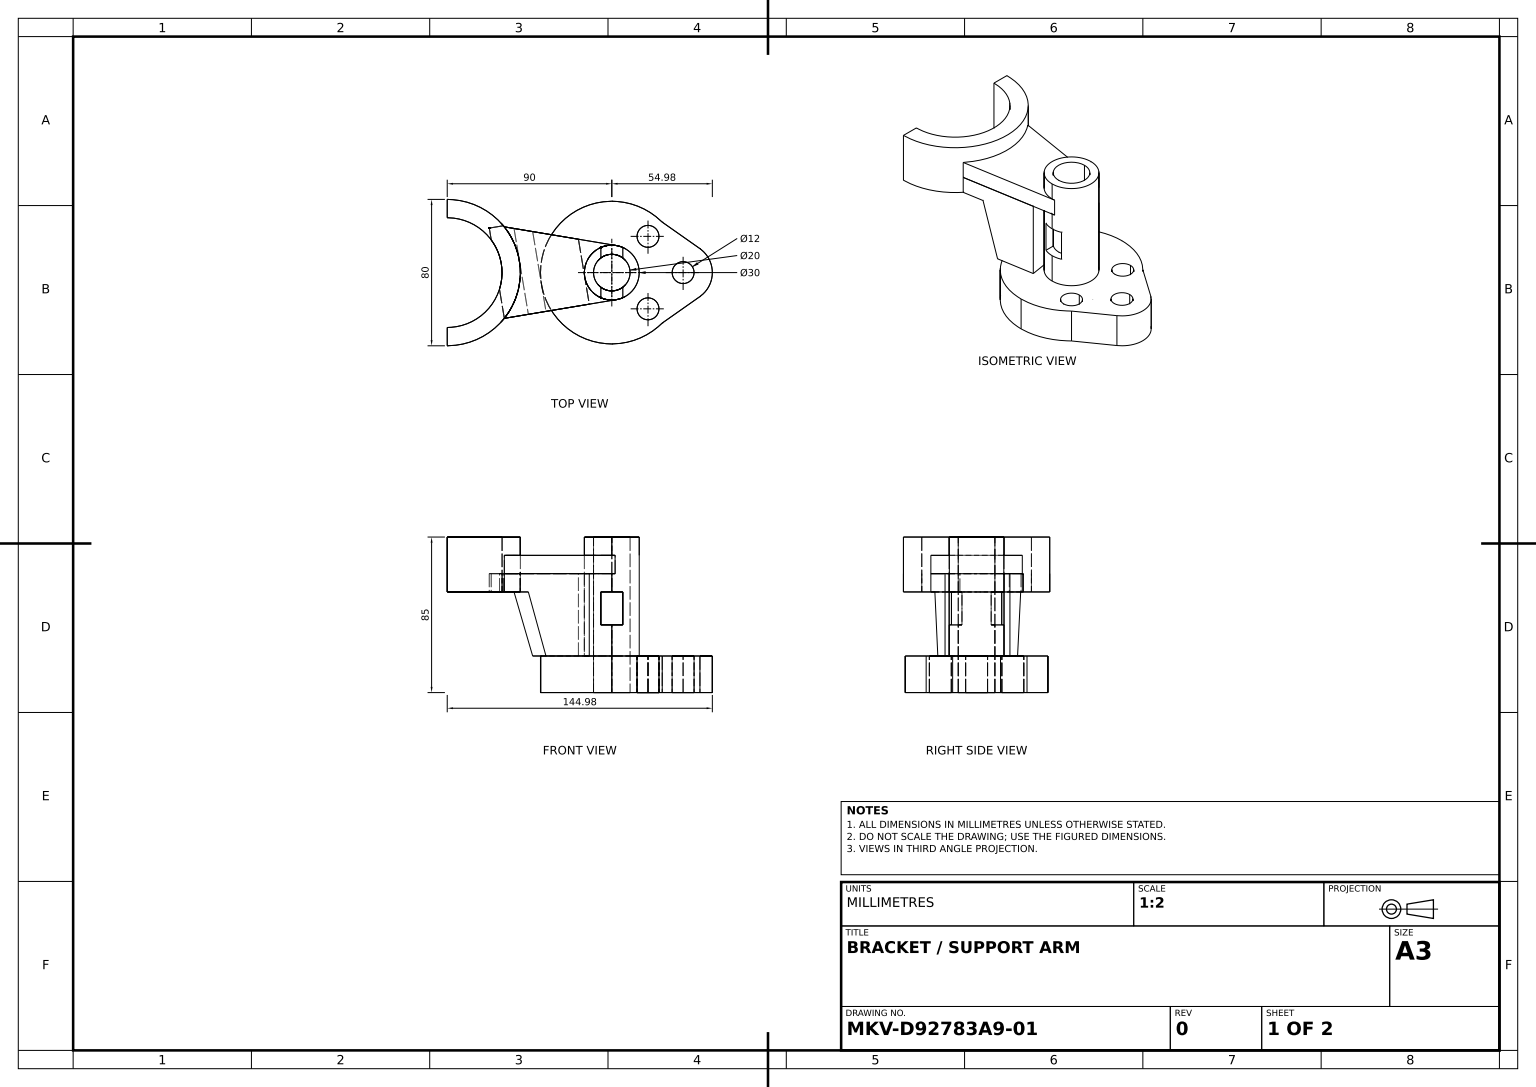
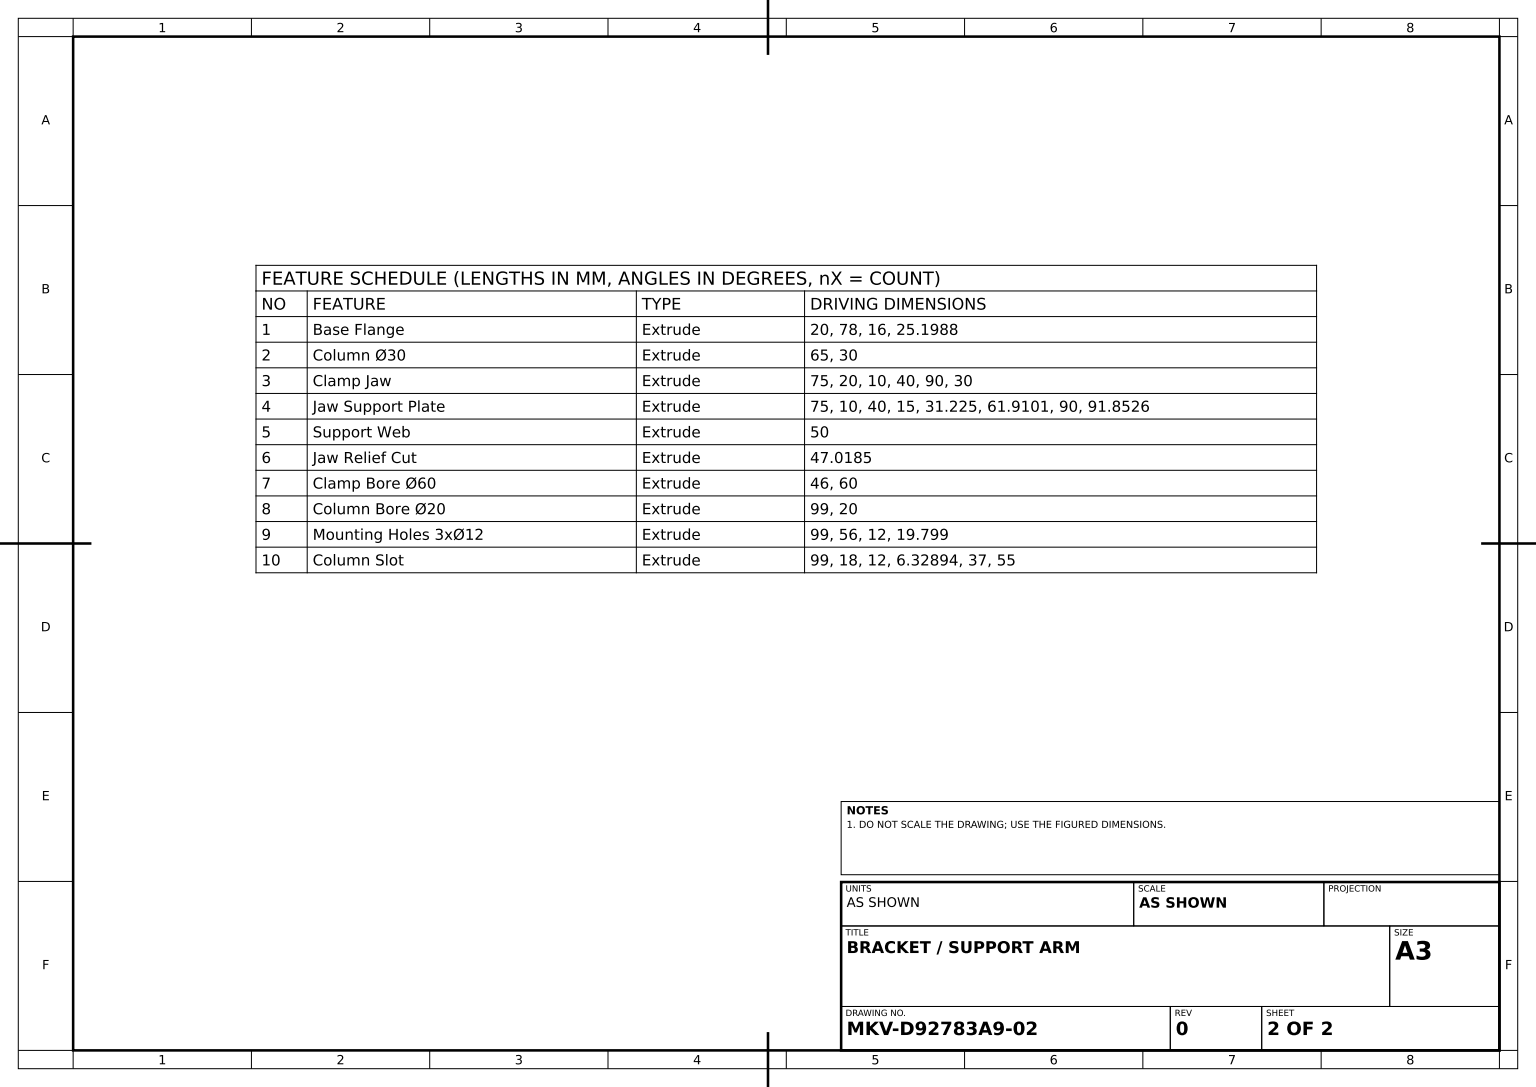
from build123d import *

# Parameters (mm, degrees)
BASE_FLANGE_DEPTH          = 20
COLUMN_SKETCH_R            = 15
COLUMN_30_DEPTH            = 65
CLAMP_JAW_DEPTH            = 10
CLAMP_JAW_DEPTH_BACK       = 20
JAW_START                  = -10
JAW_SUPPORT_PLATE_DEPTH    = 10
SUPPORT_WEB_DEPTH          = 50
JAW_START_2                = -45
JAW_RELIEF_CUT_DEPTH       = 45
CLAMP_START                = -46
CLAMP_BORE_SKETCH_R        = 30
CLAMP_BORE_60_DEPTH        = 46
COLUMN_BORE_SKETCH_R       = 10
COLUMN_BORE_20_DEPTH       = 99
MOUNTING_HOLES_SKETCH_R    = 6
MOUNTING_HOLES_3X_12_DEPTH = 99
COLUMN_SLOT_DEPTH          = 49.5


with BuildPart() as part:
    # Base Flange Sketch → Base Flange (new body)
    with BuildSketch(Plane(origin=(0, 0, 0), x_dir=(1, 0, 0), z_dir=(0, 1, 0))):
        with BuildLine():
            Line((48.196997695, 13.09256405), (27.577164466, 27.577164466))
            ThreePointArc((27.577164466, 27.577164466), (-39, 0), (27.577164466, -27.577164466))
            Line((27.577164466, -27.577164466), (48.196997695, -13.09256405))
            ThreePointArc((48.196997695, -13.09256405), (55, 0), (48.196997695, 13.09256405))
        make_face()
    extrude(amount=BASE_FLANGE_DEPTH)

    # Column Sketch → Column Ø30 (add)
    with BuildSketch(Plane(origin=(0, 20, 0), x_dir=(1, 0, 0), z_dir=(0, 1, 0))):
        with Locations(Location((0, 0, 0), (0, 0, 270))):
            Circle(COLUMN_SKETCH_R)
    extrude(amount=COLUMN_30_DEPTH)



with BuildPart() as body_2:
    # Clamp Jaw Sketch → Clamp Jaw (new, two sides: drawn at the far end of the back side and taken through both)
    with BuildSketch(Plane(origin=(0, 75, 0), x_dir=(1, 0, 0), z_dir=(0, 1, 0)).offset(-CLAMP_JAW_DEPTH_BACK)):
        with BuildLine():
            Line((-90, 30), (-90, 40))
            ThreePointArc((-90, 40), (-50, 0), (-90, -40))
            Line((-90, -40), (-90, -30))
            ThreePointArc((-90, -30), (-60, 0), (-90, 30))
        make_face()
    extrude(amount=CLAMP_JAW_DEPTH + CLAMP_JAW_DEPTH_BACK)


with BuildPart() as part_1:
    add(part.part)

    add(body_2.part)  # Jaw Support Plate merges body 2
    # Jaw Support Plate Sketch → Jaw Support Plate (add)
    with BuildSketch(Plane(origin=(0, 75, 0), x_dir=(1, 0, 0), z_dir=(0, 1, 0)).offset(JAW_START)):
        with BuildLine():
            ThreePointArc((1.852586009, 14.885157879), (-14.98589618, -0.650319682), (3.13508959, -14.668715461))
            Line((3.13508959, -14.668715461), (-58.775010008, -25))
            ThreePointArc((-58.775010008, -25), (-50, 0), (-58.775010008, 25))
            Line((-58.775010008, 25), (1.852586009, 14.885157879))
        make_face()
    extrude(amount=JAW_SUPPORT_PLATE_DEPTH)

    # Column Bore Sketch → Column Bore Ø20 (cut)
    with BuildSketch(Plane(origin=(0, 85, 0), x_dir=(1, 0, 0), z_dir=(0, 1, 0))):
        with Locations(Location((0, 0, 0), (0, 0, 270))):
            Circle(COLUMN_BORE_SKETCH_R)
    extrude(amount=-COLUMN_BORE_20_DEPTH, mode=Mode.SUBTRACT)

    # Mounting Holes Sketch → Mounting Holes 3xØ12 (cut)
    with BuildSketch(Plane(origin=(0, 20, 0), x_dir=(1, 0, 0), z_dir=(0, 1, 0))):
        with Locations(Location((39, 0, 0), (0, 0, 270))):
            Circle(MOUNTING_HOLES_SKETCH_R)
        with Locations(Location((19.798989873, 19.798989873, 0), (0, 0, 270))):
            Circle(MOUNTING_HOLES_SKETCH_R)
        with Locations(Location((19.798989873, -19.798989873, 0), (0, 0, 270))):
            Circle(MOUNTING_HOLES_SKETCH_R)
    extrude(amount=-MOUNTING_HOLES_3X_12_DEPTH, mode=Mode.SUBTRACT)

    # Column Slot Sketch → Column Slot (cut, symmetric)
    with BuildSketch(Plane.XY):
        Polygon((0, 55), (6, 55), (6, 37), (-6, 37), (-6, 55), align=None)
    extrude(amount=COLUMN_SLOT_DEPTH, both=True, mode=Mode.SUBTRACT)


with BuildPart() as body_2_2:
    # Support Web Sketch → Support Web (new body)
    with BuildSketch(Plane(origin=(2.466469942, 0, 14.78029176), x_dir=(0.9863604857263539, 0, -0.1645994902716021), z_dir=(0.1645994902716021, 0, 0.9863604857263539))):
        Polygon((-15, 20), (-15, 65), (-62.088334677, 65), (-62.088334677, 55), (-48.772443715, 55), (-39, 20), align=None)
    extrude(amount=-SUPPORT_WEB_DEPTH)

    # Jaw Relief Cut Sketch → Jaw Relief Cut (cut)
    with BuildSketch(Plane(origin=(0, 65, 0), x_dir=(1, 0, 0), z_dir=(0, 1, 0)).offset(JAW_START_2)):
        with BuildLine():
            ThreePointArc((-59.272053619, 25.608461711), (-59.02203787, 25.305451236), (-58.775010008, 25))
            Line((-58.775010008, 25), (-18.251093745, 18.239167606))
            Line((-18.251093745, 18.239167606), (-20.558911858, 32.068740172))
            Line((-20.558911858, 32.068740172), (-59.272053619, 25.608461711))
        make_face()
    extrude(amount=JAW_RELIEF_CUT_DEPTH, mode=Mode.SUBTRACT)

    # Clamp Bore Sketch → Clamp Bore Ø60 (cut)
    with BuildSketch(Plane(origin=(0, 85, 0), x_dir=(1, 0, 0), z_dir=(0, 1, 0)).offset(CLAMP_START)):
        with Locations((-90, 0)):
            Circle(CLAMP_BORE_SKETCH_R)
    extrude(amount=CLAMP_BORE_60_DEPTH, mode=Mode.SUBTRACT)


solid = Compound([part_1.part, body_2_2.part])
